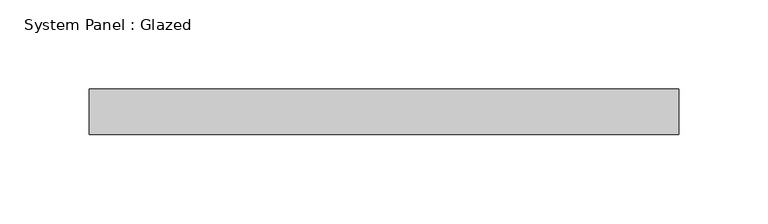
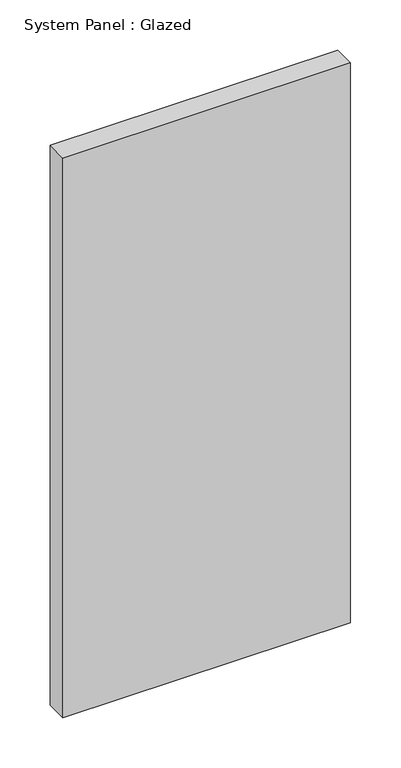
"""IFC4 building model written with IfcOpenShell, lengths in millimetres: plate geometry, System Panel : Glazed."""

from ifc_helpers import new_model, si_unit, origin, origin_with_axes, place, context, project, spatial, polyline, outline, extrude, source, transform, mapped, element, save


def system_panel_glazed_28fed175(model_context):
    return source(origin(), model_context, "Body", "SweptSolid", [
        extrude(outline(polyline([(165.1, 19.05), (-165.1, 19.05), (-165.1, 44.45), (165.1, 44.45), (165.1, 19.05)])), origin_with_axes(), (0.0, 0.0, 1.0), 680.0209318),
    ])


if __name__ == "__main__":
    model = new_model("IFC4")
    model_context = context("Model", 3, world=origin())
    ifc_project = project(units=[si_unit("LENGTHUNIT", "METRE", prefix="MILLI")], contexts=[model_context])
    site = spatial("IfcSite", under=ifc_project)
    building = spatial("IfcBuilding", under=site)
    placement = place(None, origin())
    system_panel_glazed_shape = system_panel_glazed_28fed175(model_context)
    element("IfcPlate", 1, ObjectType="System Panel : Glazed", at=placement, inside=building, context=model_context, shape_type="MappedRepresentation", body=[
        mapped(system_panel_glazed_shape, transform((0.0, 0.0, 0.0), x_axis=(1.0, 0.0, 0.0), y_axis=(0.0, 1.0, 0.0), z_axis=(0.0, 0.0, 1.0))),
    ])
    save(model, "model.ifc")

# Revit data of these elements
# Type "System Panel : Glazed"
#   Construction Type Id = "GSP4R"
#   Analytic Construction = "1/8 in Pilkington single glazing"
#   Visual Light Transmittance = 0.9
#   Solar Heat Gain Coefficient = 0.86
#   Heat Transfer Coefficient (U) = 1.18115 BTU/(h·ft²·°F)
#   Define Thermal Properties by = 1
# Element 1 (IfcPlate, "System Panel : Glazed")
#   Materials on its faces: "Glass"
# Materials
#   "Glass": class "Glass", colour RGB 0 128 192, transparency 0.75, Description = "Soda Lime Glass", Cost = 0
